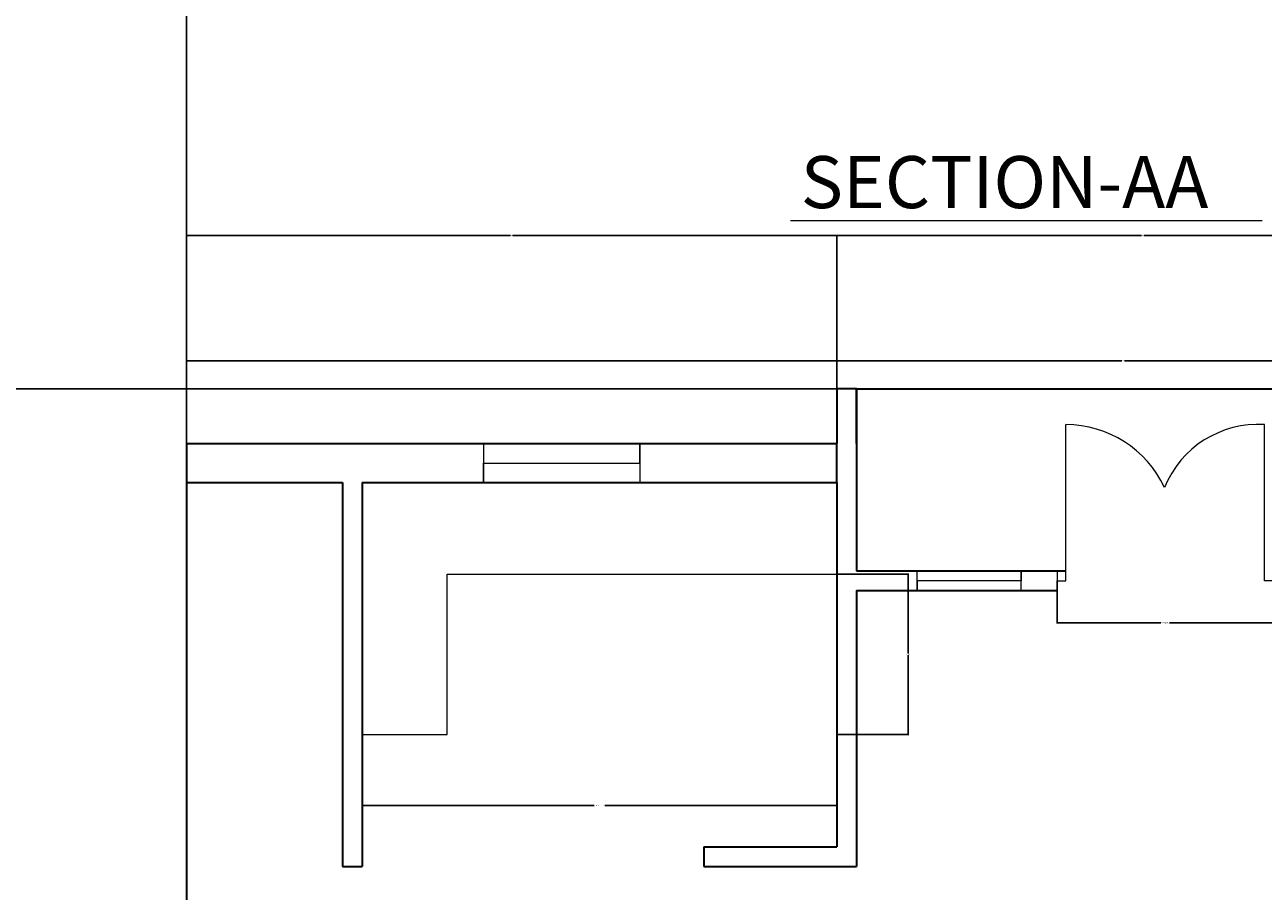
# Model space of a CAD drawing. Units: inches. Extents: x 2250 to 3547, y 1387 to 2604.
# Tile 6 of 11: x 2814 to 3100, y 2129 to 2329. Entities that reach past the tile are written whole.
import ezdxf

# ---------------------------------------------------------------- set-up
doc = ezdxf.new("R2010")
doc.units = ezdxf.units.IN
for name, color, linetype, lineweight in [('A-ANNO-DIMS', 2, 'Continuous', 18), ('A-ANNO-TEXT', 7, 'Continuous', 18), ('A-DOOR', 3, 'Continuous', 18), ('A-FLOR-CASE', 9, 'Continuous', 18), ('A-GLAZ', 4, 'Continuous', 18), ('A-WALL', 7, 'Continuous', 35)]:
    doc.layers.add(name, color=color, linetype=linetype, lineweight=lineweight)
doc.styles.get("Standard").update_dxf_attribs({"font": 'arial.ttf'})
doc.dimstyles.get("Standard").update_dxf_attribs({"dimtxt": 0.18, "dimasz": 0.18, "dimexe": 0.18, "dimexo": 0.0625, "dimgap": 0.09, "dimtad": 0, "dimtih": 1, "dimtoh": 1, "dimdec": 4, "dimzin": 0, "dimdsep": 46, "dimtxsty": 'Standard', "dimcen": 0.09, "dimadec": 0, "dimazin": 0, "dimtfac": 1, "dimtdec": 4, "dimtofl": 0, "dimtmove": 0, "dimatfit": 3, "dimfxl": 1, "dimtolj": 1, "dimtzin": 0, "dimarcsym": 0})

# ---------------------------------------------------------------- blocks, each defined once
blk = doc.blocks.new('WIN-24-SHALLOW')
for p, q in [((0, 4.5), (0, 0)), ((24, 2.25), (24, 4.5)), ((24, 4.5), (24, 0)), ((0, 0), (0, 2.25)), ((0, 2.25), (24, 2.25))]:
    blk.add_line(p, q)
blk = doc.blocks.new('WIN-36')
for p, q in [((0, 9), (0, 0)), ((36, 4.5), (36, 9)), ((36, 9), (36, 0)), ((0, 0), (0, 4.5)), ((0, 4.5), (36, 4.5))]:
    blk.add_line(p, q)
blk = doc.blocks.new('DOOR-ENTRY-DOUBLE-NORTH')
for p, q in [((2, 2.25), (2, 38.25)), ((47.76, 2.25), (47.76, 38.25)), ((0, 4.5), (0, 0)), ((49.76, 4.5), (49.76, 0)), ((0, 0), (0, 2.25)), ((0, 2.25), (2, 2.25)), ((49.76, 2.25), (47.76, 2.25)), ((49.76, 0), (49.76, 2.25))]:
    blk.add_line(p, q)
for centre, radius, start, end in [((2, 13.14), 25.11, 25.0388, 90), ((46.3, 15.04), 23.26, 86.4027, 157.9547)]:
    blk.add_arc(centre, radius, start, end)
blk = doc.blocks.new('COUNTER-KITCHEN-N')
for p, q in [((19.63, 0), (19.63, 36.95)), ((19.63, 36.95), (109.5, 36.95)), ((0, 0), (19.63, 0))]:
    blk.add_line(p, q)
blk = doc.blocks.new('*D40')
at = {"layer": 'A-ANNO-DIMS', "color": 0, "lineweight": -2, "transparency": 16777216}
for p, q in [((3052.42, 2198.61), (3052.42, 2191.03)), ((3102.18, 2198.61), (3102.18, 2191.03)), ((3052.6, 2191.21), (3076.31, 2191.21)), ((3102, 2191.21), (3078.28, 2191.21))]:
    blk.add_line(p, q, dxfattribs=at)
at = {"layer": 'A-ANNO-DIMS', "color": 0, "transparency": 16777216}
for points in [[(3052.6, 2191.24), (3052.6, 2191.18), (3052.42, 2191.21)], [(3102, 2191.24), (3102, 2191.18), (3102.18, 2191.21)]]:
    blk.add_solid(points, dxfattribs=at)
at = {"layer": 'Defpoints', "color": 0, "transparency": 16777216}
for p in [(3052.42, 2198.68), (3102.18, 2198.68), (3102.18, 2191.21)]:
    blk.add_point(p, dxfattribs=at)
at = {"layer": 'A-ANNO-DIMS', "color": 0, "transparency": 16777216, "insert": (3077.3, 2191.21), "char_height": 0.18, "attachment_point": 5}
blk.add_mtext('\\A1;ENTRY 50 TYP.', dxfattribs=at)
blk = doc.blocks.new('*D74')
at = {"layer": 'A-ANNO-DIMS', "color": 0, "lineweight": -2, "transparency": 16777216}
for p, q in [((2892.13, 2165.43), (2892.13, 2148.89)), ((3001.63, 2165.43), (3001.63, 2148.89)), ((2892.31, 2149.07), (2945.63, 2149.07)), ((3001.45, 2149.07), (2948.13, 2149.07))]:
    blk.add_line(p, q, dxfattribs=at)
at = {"layer": 'A-ANNO-DIMS', "color": 0, "transparency": 16777216}
for points in [[(2892.31, 2149.1), (2892.31, 2149.04), (2892.13, 2149.07)], [(3001.45, 2149.1), (3001.45, 2149.04), (3001.63, 2149.07)]]:
    blk.add_solid(points, dxfattribs=at)
at = {"layer": 'Defpoints', "color": 0, "transparency": 16777216}
for p in [(2892.13, 2165.49), (3001.63, 2165.49), (3001.63, 2149.07)]:
    blk.add_point(p, dxfattribs=at)
at = {"layer": 'A-ANNO-DIMS', "color": 0, "transparency": 16777216, "insert": (2946.88, 2149.07), "char_height": 0.18, "attachment_point": 5}
blk.add_mtext('\\A1;COUNTER 110 TYP.', dxfattribs=at)
blk = doc.blocks.new('*D75')
at = {"layer": 'A-ANNO-DIMS', "color": 0, "lineweight": -2, "transparency": 16777216}
for p, q in [((3001.69, 2202.45), (3018.23, 2202.45)), ((3018.05, 2202.27), (3018.05, 2184.15)), ((3018.05, 2165.67), (3018.05, 2183.79)), ((3001.69, 2165.49), (3018.23, 2165.49))]:
    blk.add_line(p, q, dxfattribs=at)
at = {"layer": 'A-ANNO-DIMS', "color": 0, "transparency": 16777216}
for points in [[(3018.02, 2202.27), (3018.08, 2202.27), (3018.05, 2202.45)], [(3018.02, 2165.67), (3018.08, 2165.67), (3018.05, 2165.49)]]:
    blk.add_solid(points, dxfattribs=at)
at = {"layer": 'Defpoints', "color": 0, "transparency": 16777216}
for p in [(3001.63, 2202.45), (3018.05, 2202.45), (3001.63, 2165.49)]:
    blk.add_point(p, dxfattribs=at)
at = {"layer": 'A-ANNO-DIMS', "color": 0, "transparency": 16777216, "insert": (3018.05, 2183.97), "char_height": 0.18, "attachment_point": 5}
blk.add_mtext('\\A1;37 TYP.', dxfattribs=at)
blk = doc.blocks.new('*D85')
at = {"layer": 'A-ANNO-DIMS', "color": 0, "lineweight": -2, "transparency": 16777216}
for p, q in [((3001.57, 2245.18), (2779.34, 2245.18)), ((2779.52, 2245), (2779.52, 1894.73)), ((2779.52, 1544.1), (2779.52, 1894.37)), ((2851.57, 1543.92), (2779.34, 1543.92))]:
    blk.add_line(p, q, dxfattribs=at)
at = {"layer": 'A-ANNO-DIMS', "color": 0, "transparency": 16777216}
for points in [[(2779.49, 2245), (2779.55, 2245), (2779.52, 2245.18)], [(2779.49, 1544.1), (2779.55, 1544.1), (2779.52, 1543.92)]]:
    blk.add_solid(points, dxfattribs=at)
at = {"layer": 'Defpoints', "color": 0, "transparency": 16777216}
for p in [(2779.52, 2245.18), (3001.63, 2245.18), (2851.63, 1543.92)]:
    blk.add_point(p, dxfattribs=at)
at = {"layer": 'A-ANNO-DIMS', "color": 0, "transparency": 16777216, "insert": (2779.52, 1894.55), "char_height": 0.18, "attachment_point": 5}
blk.add_mtext('\\A1;701.3', dxfattribs=at)
blk = doc.blocks.new('*D92')
at = {"layer": 'A-ANNO-DIMS', "color": 0, "lineweight": -2, "transparency": 16777216}
for p, q in [((2851.63, 2232.63), (2851.63, 2280.71)), ((2851.81, 2280.53), (2926.35, 2280.53)), ((3001.45, 2280.53), (2926.91, 2280.53)), ((3001.63, 2245.24), (3001.63, 2280.71))]:
    blk.add_line(p, q, dxfattribs=at)
at = {"layer": 'A-ANNO-DIMS', "color": 0, "transparency": 16777216}
for points in [[(2851.81, 2280.56), (2851.81, 2280.5), (2851.63, 2280.53)], [(3001.45, 2280.56), (3001.45, 2280.5), (3001.63, 2280.53)]]:
    blk.add_solid(points, dxfattribs=at)
at = {"layer": 'Defpoints', "color": 0, "transparency": 16777216}
for p in [(3001.63, 2280.53), (3001.63, 2245.18), (2851.63, 2232.56)]:
    blk.add_point(p, dxfattribs=at)
at = {"layer": 'A-ANNO-DIMS', "color": 0, "transparency": 16777216, "insert": (2926.63, 2280.53), "char_height": 0.18, "attachment_point": 5}
blk.add_mtext('\\A1;150', dxfattribs=at)
blk = doc.blocks.new('*D93')
at = {"layer": 'A-ANNO-DIMS', "color": 0, "lineweight": -2, "transparency": 16777216}
for p, q in [((3001.63, 2245.24), (3001.63, 2280.71)), ((3001.81, 2280.53), (3071.87, 2280.53)), ((3142.45, 2280.53), (3072.39, 2280.53)), ((3142.63, 2245.24), (3142.63, 2280.71))]:
    blk.add_line(p, q, dxfattribs=at)
at = {"layer": 'A-ANNO-DIMS', "color": 0, "transparency": 16777216}
for points in [[(3001.81, 2280.56), (3001.81, 2280.5), (3001.63, 2280.53)], [(3142.45, 2280.56), (3142.45, 2280.5), (3142.63, 2280.53)]]:
    blk.add_solid(points, dxfattribs=at)
at = {"layer": 'Defpoints', "color": 0, "transparency": 16777216}
for p in [(3142.63, 2280.53), (3001.63, 2245.18), (3142.63, 2245.18)]:
    blk.add_point(p, dxfattribs=at)
at = {"layer": 'A-ANNO-DIMS', "color": 0, "transparency": 16777216, "insert": (3072.13, 2280.53), "char_height": 0.18, "attachment_point": 5}
blk.add_mtext('\\A1;141', dxfattribs=at)
blk = doc.blocks.new('*D108')
at = {"layer": 'A-ANNO-DIMS', "color": 0, "lineweight": -2, "transparency": 16777216}
for p, q in [((2851.63, 2333.89), (2851.63, 2251.45)), ((3283.63, 2333.89), (3283.63, 2251.45)), ((2851.81, 2251.63), (3067.34, 2251.63)), ((3283.45, 2251.63), (3067.92, 2251.63))]:
    blk.add_line(p, q, dxfattribs=at)
at = {"layer": 'A-ANNO-DIMS', "color": 0, "transparency": 16777216}
for points in [[(2851.81, 2251.66), (2851.81, 2251.6), (2851.63, 2251.63)], [(3283.45, 2251.66), (3283.45, 2251.6), (3283.63, 2251.63)]]:
    blk.add_solid(points, dxfattribs=at)
at = {"layer": 'Defpoints', "color": 0, "transparency": 16777216}
for p in [(2851.63, 2333.95), (3283.63, 2333.95), (3283.63, 2251.63)]:
    blk.add_point(p, dxfattribs=at)
at = {"layer": 'A-ANNO-DIMS', "color": 0, "transparency": 16777216, "insert": (3067.63, 2251.63), "char_height": 0.18, "attachment_point": 5}
blk.add_mtext('\\A1;432', dxfattribs=at)

msp = doc.modelspace()

# ---------------------------------------------------------------- linework, layer by layer
at = {"layer": 'A-ANNO-TEXT'}
msp.add_line((2990.9226, 2283.981), (3099.6644, 2283.981), dxfattribs=at)
at = {"layer": 'A-WALL'}
for p, q in [((3006.1288, 2245.1762), (3001.6288, 2245.1762)), ((3001.6288, 2245.1762), (3001.6288, 2232.5639)), ((3006.1288, 2245.1762), (3006.1288, 2203.1762)), ((3006.1288, 2232.5639), (3006.1288, 2245.1762)), ((3006.1288, 2245.1762), (3138.1288, 2245.1762)), ((2851.6288, 2232.5639), (2851.6288, 1899.5639)), ((2851.6288, 2232.5639), (2851.6288, 1899.5639)), ((2851.6288, 2232.5639), (3001.6288, 2232.5639)), ((3001.6288, 2223.5639), (3001.6288, 2232.5639)), ((2851.6288, 2223.5639), (2887.6288, 2223.5639)), ((2887.6288, 2223.5639), (2887.6288, 2135.0639)), ((2892.1288, 2223.5639), (2892.1288, 2135.0639)), ((2892.1288, 2223.5639), (3001.6288, 2223.5639)), ((3001.6288, 2223.5639), (3001.6288, 2139.5639)), ((3006.1288, 2203.1762), (3054.4171, 2203.1762)), ((3006.1288, 2198.6762), (3006.1288, 2135.0639)), ((3006.1288, 2198.6762), (3052.4171, 2198.6762)), ((2970.9285, 2139.5639), (3001.6288, 2139.5639)), ((2970.9285, 2139.5639), (2970.9285, 2135.0639)), ((2887.6288, 2135.0639), (2892.1288, 2135.0639)), ((2970.9285, 2135.0639), (3006.1288, 2135.0639))]:
    msp.add_line(p, q, dxfattribs=at)

# ---------------------------------------------------------------- block references
at = {"layer": 'A-DOOR'}
msp.add_blockref('DOOR-ENTRY-DOUBLE-NORTH', (3052.4171, 2198.6762), dxfattribs=at)
at = {"layer": 'A-FLOR-CASE'}
msp.add_blockref('COUNTER-KITCHEN-N', (2892.1288, 2165.4936), dxfattribs=at)
at = {"layer": 'A-GLAZ'}
msp.add_blockref('WIN-36', (2920.1441, 2223.5639), dxfattribs=at)
at = {"layer": 'A-GLAZ', "rotation": 180}
msp.add_blockref('WIN-24-SHALLOW', (3044.1287, 2203.1762), dxfattribs=at)

# ---------------------------------------------------------------- texts
at = {"layer": 'A-ANNO-TEXT', "insert": (2993.2647, 2298.857), "char_height": 12, "attachment_point": 1}
msp.add_mtext_dynamic_manual_height_columns('SECTION-AA', width=308.899708, gutter_width=12.5, heights=[0], dxfattribs=at)

# ---------------------------------------------------------------- dimensions: what is measured, and where the dimension line sits
at = {"layer": 'A-ANNO-DIMS'}
for base, p1, p2, picture, middle in [((3283.6288, 2251.631), (2851.6288, 2333.9493), (3283.6288, 2333.9493), '*D108', (3067.6288, 2251.631)), ((3001.6288, 2280.5262), (2851.6288, 2232.5639), (3001.6288, 2245.1762), '*D92', (2926.6288, 2280.5262)), ((3142.6288, 2280.5262), (3001.6288, 2245.1762), (3142.6288, 2245.1762), '*D93', (3072.1288, 2280.5262))]:
    dim = msp.add_linear_dim(base=base, p1=p1, p2=p2, dimstyle='Standard', override={"dimdec": 0, "dimlfac": 1, "dimrnd": 0, "dimzin": 0, "dimdsep": 46, "dimlunit": 2}, dxfattribs=at)
    dim.commit()
    dim.dimension.update_dxf_attribs({"geometry": picture, "text_midpoint": middle})
dim = msp.add_linear_dim(base=(2779.5165, 2245.1762), p1=(2851.6288, 1543.9245), p2=(3001.6288, 2245.1762), angle=90, dimstyle='Standard', override={"dimdec": 1, "dimlfac": 1, "dimrnd": 0, "dimzin": 0, "dimdsep": 46, "dimlunit": 2}, dxfattribs=at)
dim.commit()
dim.dimension.update_dxf_attribs({"geometry": '*D85', "text_midpoint": (2779.5165, 1894.5504)})
dim = msp.add_linear_dim(base=(3018.0538, 2202.4485), p1=(3001.6288, 2165.4936), p2=(3001.6288, 2202.4485), angle=90, text='<> TYP.', dimstyle='Standard', override={"dimdec": 0, "dimlfac": 1, "dimrnd": 0, "dimzin": 0, "dimdsep": 46, "dimlunit": 2}, dxfattribs=at)
dim.commit()
dim.dimension.update_dxf_attribs({"geometry": '*D75', "text_midpoint": (3018.0538, 2183.9711)})
for base, p1, p2, text, picture, middle in [((3102.1799, 2191.2118), (3052.4171, 2198.6762), (3102.1799, 2198.6762), 'ENTRY <> TYP.', '*D40', (3077.2985, 2191.2118)), ((3001.6287612161, 2149.0685789044), (2892.1287612161, 2165.4935789044), (3001.6287612161, 2165.4935789044), 'COUNTER <> TYP.', '*D74', (2946.8787612161, 2149.0685789044))]:
    dim = msp.add_linear_dim(base=base, p1=p1, p2=p2, text=text, dimstyle='Standard', override={"dimdec": 0, "dimlfac": 1, "dimrnd": 0, "dimzin": 0, "dimdsep": 46, "dimlunit": 2}, dxfattribs=at)
    dim.commit()
    dim.dimension.update_dxf_attribs({"geometry": picture, "text_midpoint": middle})

doc.saveas('drawing.dxf')
